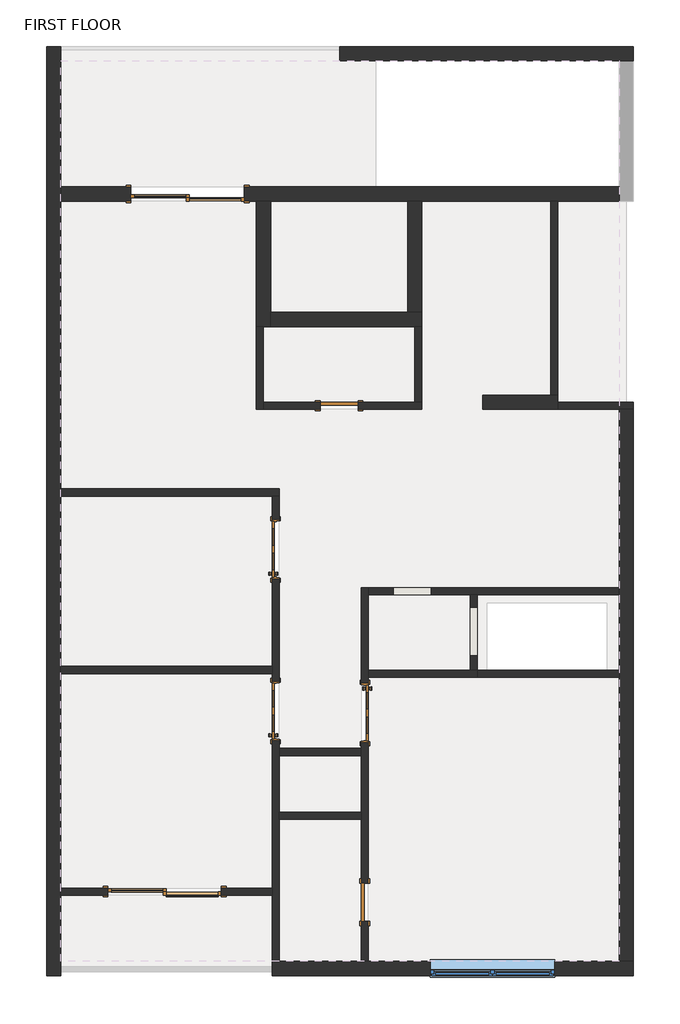
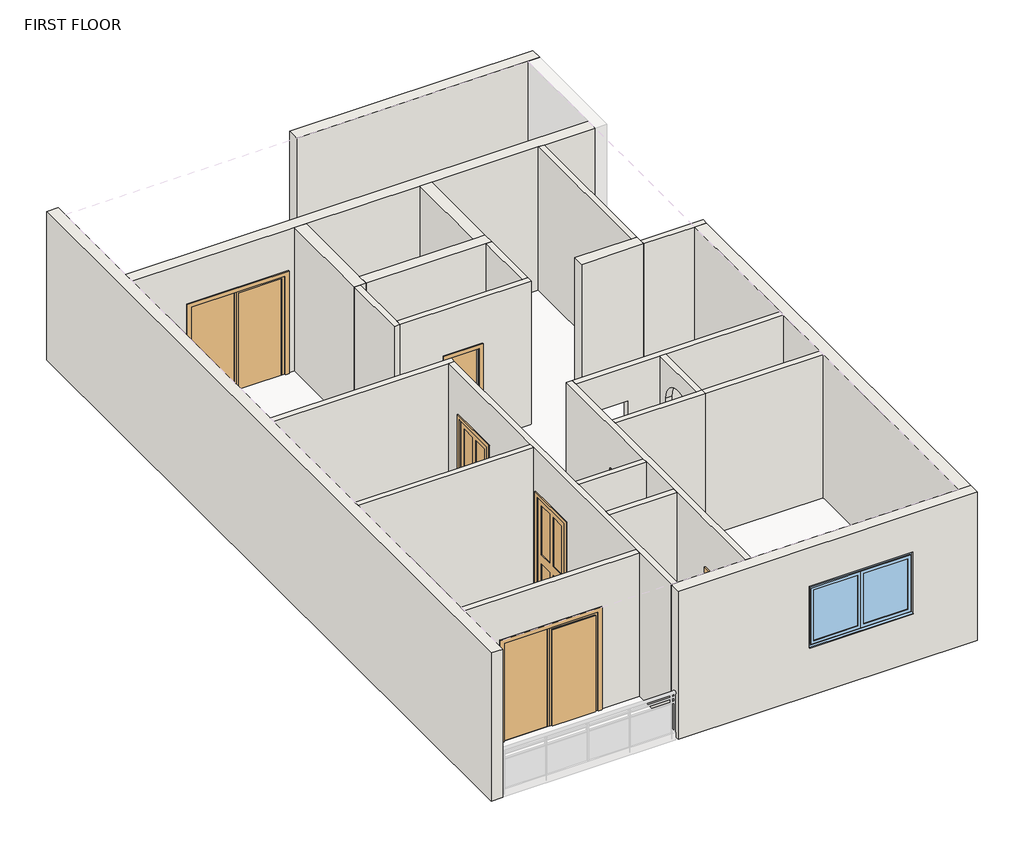
# One storey, part 1 of 2: 25 walls, 7 doors, 1 window.
"""IFC4 building model written with IfcOpenShell, lengths in millimetres."""

from ifc_helpers import new_model, si_unit, point, frame, frame_2d, origin, place, context, project, spatial, polyline, circle_curve, trimmed, segment, composite_curve, outline, extrude, faceted_brep, transform, mapped, element, save
from components import door_d4d75d1e, door_166d4031, door_c2926031, single_flush_bathroom_door_2_x_7_d2bb450e, w2_w2_7b90d420

model = new_model("IFC4")

# Units and contexts
model_context = context("Model", 3, world=origin())
ifc_project = project(units=[si_unit("LENGTHUNIT", "METRE", prefix="MILLI")], contexts=[model_context])

# Site, building, storey
site = spatial("IfcSite", under=ifc_project)
building = spatial("IfcBuilding", under=site)
storey = spatial("IfcBuildingStorey", under=building, Name="FIRST FLOOR", Elevation=3352.8)

# Doors
placement = place(None, origin())
door_shape = door_d4d75d1e(model_context)
element("IfcDoor", 1, ObjectType="Door-Double-Sliding : 72\" x 84\"", at=placement, inside=storey, context=model_context, shape_type="MappedRepresentation", body=[
    mapped(door_shape, transform((-16100.4229553, 5649.1964313, 3352.8), x_axis=(-1.0, 0.0, 0.0), y_axis=(0.0, -1.0, 0.0), z_axis=(0.0, 0.0, 1.0))),
])
door_2_shape = door_166d4031(model_context)
element("IfcDoor", 2, ObjectType="Door-Double-Sliding : 72\" x 84\"", at=placement, inside=storey, context=model_context, shape_type="MappedRepresentation", body=[
    mapped(door_2_shape, transform((-16471.8979553, -5583.9535687, 3352.8), x_axis=(-1.0, 0.0, 0.0), y_axis=(0.0, -1.0, 0.0), z_axis=(0.0, 0.0, 1.0))),
])
door_3_shape = door_c2926031(model_context)
element("IfcDoor", 3, ObjectType="Door-Interior-Single-4_Panel-Wood : 36\" x 84\"", at=placement, inside=storey, context=model_context, shape_type="MappedRepresentation", body=[
    mapped(door_3_shape, transform((-13246.0979553, -2834.4035687, 3352.8), x_axis=(0.0, -1.0, 0.0), y_axis=(1.0, 0.0, 0.0), z_axis=(0.0, 0.0, 1.0))),
])
element("IfcDoor", 4, ObjectType="Door-Interior-Single-4_Panel-Wood : 36\" x 84\"", at=placement, inside=storey, context=model_context, shape_type="MappedRepresentation", body=[
    mapped(door_3_shape, transform((-14687.5479553, -199.1535687, 3352.8), x_axis=(0.0, 1.0, 0.0), y_axis=(-1.0, 0.0, 0.0), z_axis=(0.0, 0.0, 1.0))),
])
element("IfcDoor", 5, ObjectType="Door-Interior-Single-4_Panel-Wood : 36\" x 84\"", at=placement, inside=storey, context=model_context, shape_type="MappedRepresentation", body=[
    mapped(door_3_shape, transform((-14687.5479553, -2802.6535687, 3352.8), x_axis=(0.0, 1.0, 0.0), y_axis=(-1.0, 0.0, 0.0), z_axis=(0.0, 0.0, 1.0))),
])
single_flush_bathroom_door_2_x_7_shape = single_flush_bathroom_door_2_x_7_d2bb450e(model_context)
element("IfcDoor", 6, ObjectType="Single-Flush : BATHROOM DOOR 2' X 7'", at=placement, inside=storey, context=model_context, shape_type="MappedRepresentation", body=[
    mapped(single_flush_bathroom_door_2_x_7_shape, transform((-13249.2729553, -5882.4035687, 3352.8), x_axis=(0.0, 1.0, 0.0), y_axis=(-1.0, 0.0, 0.0), z_axis=(0.0, 0.0, 1.0))),
])
element("IfcDoor", 7, ObjectType="Single-Flush : BATHROOM DOOR 2' X 7'", at=placement, inside=storey, context=model_context, shape_type="MappedRepresentation", body=[
    mapped(single_flush_bathroom_door_2_x_7_shape, transform((-13662.0229553, 2112.2464313, 3352.8), x_axis=(1.0, 0.0, 0.0), y_axis=(0.0, 1.0, 0.0), z_axis=(0.0, 0.0, 1.0))),
])

# Walls
element("IfcWall", 8, ObjectType="EXTERIOR WALL 9\"", at=placement, inside=storey, context=model_context, shape_type="Brep", body=[
    faceted_brep([(-13649.3229553, 7668.4964313, 3352.8), (-9153.5229553, 7668.4964313, 3352.8), (-8924.9229553, 7668.4964313, 3352.8), (-8924.9229553, 7668.4964313, 6400.8), (-9153.5229553, 7668.4964313, 6400.8), (-13649.3229553, 7668.4964313, 6400.8), (-13649.3229553, 7897.0964313, 3352.8), (-13649.3229553, 7897.0964313, 6400.8), (-8924.9229553, 7897.0964313, 6400.8), (-8924.9229553, 7897.0964313, 3352.8)], [[[0, 1, 2, 3, 4, 5]], [[6, 7, 8, 9]], [[2, 1, 0, 6, 9]], [[5, 4, 3, 8, 7]], [[0, 5, 7, 6]], [[3, 2, 9, 8]]]),
])
element("IfcWall", 9, ObjectType="EXTERIOR WALL 9\"", at=placement, inside=storey, context=model_context, shape_type="Brep", body=[
    faceted_brep([(-18373.7229553, 7897.0964313, 3352.8), (-18373.7229553, -7063.5035687, 3352.8), (-18373.7229553, -7063.5035687, 6400.8), (-18373.7229553, 7897.0964313, 6400.8), (-18145.1229553, 7897.0964313, 3352.8), (-18145.1229553, 7897.0964313, 6400.8), (-18145.1229553, 5636.4964313, 6400.8), (-18145.1229553, 5407.8964313, 6400.8), (-18145.1229553, 772.3964313, 6400.8), (-18145.1229553, 658.0964313, 6400.8), (-18145.1229553, -2085.1035687, 6400.8), (-18145.1229553, -2199.4035687, 6400.8), (-18145.1229553, -5653.8035687, 6400.8), (-18145.1229553, -5768.1035687, 6400.8), (-18145.1229553, -7063.5035687, 6400.8), (-18145.1229553, -7063.5035687, 3352.8), (-18145.1229553, -5768.1035687, 3352.8), (-18145.1229553, -5653.8035687, 3352.8), (-18145.1229553, -2199.4035687, 3352.8), (-18145.1229553, -2085.1035687, 3352.8), (-18145.1229553, 658.0964313, 3352.8), (-18145.1229553, 772.3964313, 3352.8), (-18145.1229553, 5407.8964313, 3352.8), (-18145.1229553, 5636.4964313, 3352.8)], [[[0, 1, 2, 3]], [[4, 5, 6, 7, 8, 9, 10, 11, 12, 13, 14, 15, 16, 17, 18, 19, 20, 21, 22, 23]], [[1, 0, 4, 23, 22, 21, 20, 19, 18, 17, 16, 15]], [[2, 1, 15, 14]], [[3, 2, 14, 13, 12, 11, 10, 9, 8, 7, 6, 5]], [[0, 3, 5, 4]]]),
])
element("IfcWall", 10, ObjectType="EXTERIOR WALL 9\"", at=placement, inside=storey, context=model_context, shape_type="Brep", body=[
    faceted_brep([(-18145.1229553, 5407.8964313, 3352.8), (-17014.8229553, 5407.8964313, 3352.8), (-17014.8229553, 5407.8964313, 5486.4), (-15186.0229553, 5407.8964313, 5486.4), (-15186.0229553, 5407.8964313, 3352.8), (-14995.5229553, 5407.8964313, 3352.8), (-14766.9229553, 5407.8964313, 3352.8), (-12557.1229553, 5407.8964313, 3352.8), (-12328.5229553, 5407.8964313, 3352.8), (-10258.4229553, 5407.8964313, 3352.8), (-10144.1229553, 5407.8964313, 3352.8), (-9153.5229553, 5407.8964313, 3352.8), (-9153.5229553, 5407.8964313, 6400.8), (-10144.1229553, 5407.8964313, 6400.8), (-10258.4229553, 5407.8964313, 6400.8), (-12328.5229553, 5407.8964313, 6400.8), (-12557.1229553, 5407.8964313, 6400.8), (-14766.9229553, 5407.8964313, 6400.8), (-14995.5229553, 5407.8964313, 6400.8), (-18145.1229553, 5407.8964313, 6400.8), (-17014.8229553, 5636.4964313, 5486.4), (-17014.8229553, 5636.4964313, 3352.8), (-18145.1229553, 5636.4964313, 3352.8), (-18145.1229553, 5636.4964313, 6400.8), (-9153.5229553, 5636.4964313, 6400.8), (-9153.5229553, 5636.4964313, 3352.8), (-15186.0229553, 5636.4964313, 3352.8), (-15186.0229553, 5636.4964313, 5486.4)], [[[0, 1, 2, 3, 4, 5, 6, 7, 8, 9, 10, 11, 12, 13, 14, 15, 16, 17, 18, 19]], [[20, 21, 22, 23, 24, 25, 26, 27]], [[26, 25, 11, 10, 9, 8, 7, 6, 5, 4]], [[22, 21, 1, 0]], [[19, 18, 17, 16, 15, 14, 13, 12, 24, 23]], [[12, 11, 25, 24]], [[0, 19, 23, 22]], [[4, 3, 27, 26]], [[2, 1, 21, 20]], [[3, 2, 20, 27]]]),
])
element("IfcWall", 11, ObjectType="EXTERIOR WALL 9\"", at=placement, inside=storey, context=model_context, shape_type="Brep", body=[
    faceted_brep([(-14995.5229553, 5407.8964313, 3352.8), (-14995.5229553, 3388.5964313, 3352.8), (-14995.5229553, 3388.5964313, 6400.8), (-14995.5229553, 5407.8964313, 6400.8), (-14766.9229553, 5407.8964313, 3352.8), (-14766.9229553, 5407.8964313, 6400.8), (-14766.9229553, 3617.1964313, 6400.8), (-14766.9229553, 3388.5964313, 6400.8), (-14766.9229553, 3388.5964313, 3352.8), (-14766.9229553, 3617.1964313, 3352.8), (-14881.2229553, 3388.5964313, 3352.8), (-14881.2229553, 3388.5964313, 6400.8)], [[[0, 1, 2, 3]], [[4, 5, 6, 7, 8, 9]], [[1, 0, 4, 9, 8, 10]], [[3, 2, 11, 7, 6, 5]], [[0, 3, 5, 4]], [[2, 1, 10, 8, 7, 11]]]),
])
element("IfcWall", 12, ObjectType="EXTERIOR WALL 9\"", at=placement, inside=storey, context=model_context, shape_type="Brep", body=[
    faceted_brep([(-14766.9229553, 3388.5964313, 3352.8), (-12442.8229553, 3388.5964313, 3352.8), (-12328.5229553, 3388.5964313, 3352.8), (-12328.5229553, 3388.5964313, 6400.8), (-12442.8229553, 3388.5964313, 6400.8), (-14766.9229553, 3388.5964313, 6400.8), (-14766.9229553, 3617.1964313, 3352.8), (-14766.9229553, 3617.1964313, 6400.8), (-12557.1229553, 3617.1964313, 6400.8), (-12328.5229553, 3617.1964313, 6400.8), (-12328.5229553, 3617.1964313, 3352.8), (-12557.1229553, 3617.1964313, 3352.8)], [[[0, 1, 2, 3, 4, 5]], [[6, 7, 8, 9, 10, 11]], [[2, 1, 0, 6, 11, 10]], [[5, 4, 3, 9, 8, 7]], [[0, 5, 7, 6]], [[3, 2, 10, 9]]]),
])
element("IfcWall", 13, ObjectType="EXTERIOR WALL 9\"", at=placement, inside=storey, context=model_context, shape_type="SweptSolid", body=[
    extrude(outline(polyline([(-12328.5229553, 5407.8964313), (-12328.5229553, 3617.1964313), (-12557.1229553, 3617.1964313), (-12557.1229553, 5407.8964313), (-12328.5229553, 5407.8964313)])), frame((0.0, 0.0, 3352.8), z_axis=(0.0, 0.0, 1.0), x_axis=(1.0, 0.0, 0.0)), (0.0, 0.0, 1.0), 3048.0),
])
element("IfcWall", 14, ObjectType="EXTERIOR WALL 9\"", at=placement, inside=storey, context=model_context, shape_type="Brep", body=[
    faceted_brep([(-14741.5229553, -7063.5035687, 3352.8), (-8924.9229553, -7063.5035687, 3352.8), (-8924.9229553, -7063.5035687, 6400.8), (-14741.5229553, -7063.5035687, 6400.8), (-12196.8729553, -7063.5035687, 4352.8), (-12196.8729553, -7063.5035687, 5612.8), (-10186.8729553, -7063.5035687, 5612.8), (-10186.8729553, -7063.5035687, 4352.8), (-14741.5229553, -6834.9035687, 3352.8), (-14741.5229553, -6834.9035687, 6400.8), (-14627.2229553, -6834.9035687, 6400.8), (-13306.4229553, -6834.9035687, 6400.8), (-13192.1229553, -6834.9035687, 6400.8), (-9153.5229553, -6834.9035687, 6400.8), (-8924.9229553, -6834.9035687, 6400.8), (-8924.9229553, -6834.9035687, 3352.8), (-9153.5229553, -6834.9035687, 3352.8), (-13192.1229553, -6834.9035687, 3352.8), (-13306.4229553, -6834.9035687, 3352.8), (-14627.2229553, -6834.9035687, 3352.8), (-12196.8729553, -6834.9035687, 4352.8), (-10186.8729553, -6834.9035687, 4352.8), (-10186.8729553, -6834.9035687, 5612.8), (-12196.8729553, -6834.9035687, 5612.8)], [[[0, 1, 2, 3], [4, 5, 6, 7]], [[8, 9, 10, 11, 12, 13, 14, 15, 16, 17, 18, 19], [20, 21, 22, 23]], [[1, 0, 8, 19, 18, 17, 16, 15]], [[3, 2, 14, 13, 12, 11, 10, 9]], [[2, 1, 15, 14]], [[0, 3, 9, 8]], [[5, 4, 20, 23]], [[6, 5, 23, 22]], [[7, 6, 22, 21]], [[4, 7, 21, 20]]]),
])
element("IfcWall", 15, ObjectType="EXTERIOR WALL 9\"", at=placement, inside=storey, context=model_context, shape_type="Brep", body=[
    faceted_brep([(-8924.9229553, -6834.9035687, 3352.8), (-8924.9229553, 2055.0964313, 3352.8), (-8924.9229553, 2055.0964313, 6400.8), (-8924.9229553, -6834.9035687, 6400.8), (-9153.5229553, -6834.9035687, 3352.8), (-9153.5229553, -6834.9035687, 6400.8), (-9153.5229553, -2262.9035687, 6400.8), (-9153.5229553, -2148.6035687, 6400.8), (-9153.5229553, -929.4035687, 6400.8), (-9153.5229553, -815.1035687, 6400.8), (-9153.5229553, 2055.0964313, 6400.8), (-9153.5229553, 2055.0964313, 3352.8), (-9153.5229553, -815.1035687, 3352.8), (-9153.5229553, -929.4035687, 3352.8), (-9153.5229553, -2148.6035687, 3352.8), (-9153.5229553, -2262.9035687, 3352.8)], [[[0, 1, 2, 3]], [[4, 5, 6, 7, 8, 9, 10, 11, 12, 13, 14, 15]], [[1, 0, 4, 15, 14, 13, 12, 11]], [[3, 2, 10, 9, 8, 7, 6, 5]], [[0, 3, 5, 4]], [[2, 1, 11, 10]]]),
])
element("IfcWall", 16, ObjectType="EXTERIOR WALL 9\"", at=placement, inside=storey, context=model_context, shape_type="Brep", body=[
    faceted_brep([(-11350.6229553, 2055.0964313, 3352.8), (-10144.1229553, 2055.0964313, 3352.8), (-10144.1229553, 2055.0964313, 6400.8), (-11350.6229553, 2055.0964313, 6400.8), (-11350.6229553, 2283.6964313, 3352.8), (-11350.6229553, 2283.6964313, 6400.8), (-10258.4229553, 2283.6964313, 6400.8), (-10144.1229553, 2283.6964313, 6400.8), (-10144.1229553, 2283.6964313, 3352.8), (-10258.4229553, 2283.6964313, 3352.8), (-10144.1229553, 2169.3964313, 3352.8), (-10144.1229553, 2169.3964313, 6400.8)], [[[0, 1, 2, 3]], [[4, 5, 6, 7, 8, 9]], [[1, 0, 4, 9, 8, 10]], [[3, 2, 11, 7, 6, 5]], [[0, 3, 5, 4]], [[2, 1, 10, 8, 7, 11]]]),
])
element("IfcWall", 17, ObjectType="INTERIOR WALL 4.5\"", at=placement, inside=storey, context=model_context, shape_type="Brep", body=[
    faceted_brep([(-18145.1229553, 658.0964313, 3352.8), (-14741.5229553, 658.0964313, 3352.8), (-14627.2229553, 658.0964313, 3352.8), (-14627.2229553, 658.0964313, 6400.8), (-14741.5229553, 658.0964313, 6400.8), (-18145.1229553, 658.0964313, 6400.8), (-18145.1229553, 772.3964313, 3352.8), (-18145.1229553, 772.3964313, 6400.8), (-14627.2229553, 772.3964313, 6400.8), (-14627.2229553, 772.3964313, 3352.8)], [[[0, 1, 2, 3, 4, 5]], [[6, 7, 8, 9]], [[2, 1, 0, 6, 9]], [[5, 4, 3, 8, 7]], [[0, 5, 7, 6]], [[3, 2, 9, 8]]]),
])
element("IfcWall", 18, ObjectType="INTERIOR WALL 4.5\"", at=placement, inside=storey, context=model_context, shape_type="Brep", body=[
    faceted_brep([(-14741.5229553, -6834.9035687, 6400.8), (-14741.5229553, -5768.1035687, 6400.8), (-14741.5229553, -5653.8035687, 6400.8), (-14741.5229553, -2199.4035687, 6400.8), (-14741.5229553, -2085.1035687, 6400.8), (-14741.5229553, 658.0964313, 6400.8), (-14741.5229553, 658.0964313, 3352.8), (-14741.5229553, 283.4464313, 3352.8), (-14741.5229553, 283.4464313, 5511.8), (-14741.5229553, -681.7535687, 5511.8), (-14741.5229553, -681.7535687, 3352.8), (-14741.5229553, -2085.1035687, 3352.8), (-14741.5229553, -2199.4035687, 3352.8), (-14741.5229553, -2320.0535687, 3352.8), (-14741.5229553, -2320.0535687, 5511.8), (-14741.5229553, -3285.2535687, 5511.8), (-14741.5229553, -3285.2535687, 3352.8), (-14741.5229553, -5653.8035687, 3352.8), (-14741.5229553, -5768.1035687, 3352.8), (-14741.5229553, -6834.9035687, 3352.8), (-14627.2229553, 658.0964313, 6400.8), (-14627.2229553, -3405.9035687, 6400.8), (-14627.2229553, -3520.2035687, 6400.8), (-14627.2229553, -4434.6035687, 6400.8), (-14627.2229553, -4548.9035687, 6400.8), (-14627.2229553, -6834.9035687, 6400.8), (-14627.2229553, -6834.9035687, 3352.8), (-14627.2229553, -4548.9035687, 3352.8), (-14627.2229553, -4434.6035687, 3352.8), (-14627.2229553, -3520.2035687, 3352.8), (-14627.2229553, -3405.9035687, 3352.8), (-14627.2229553, -3285.2535687, 3352.8), (-14627.2229553, -3285.2535687, 5511.8), (-14627.2229553, -2320.0535687, 5511.8), (-14627.2229553, -2320.0535687, 3352.8), (-14627.2229553, -681.7535687, 3352.8), (-14627.2229553, -681.7535687, 5511.8), (-14627.2229553, 283.4464313, 5511.8), (-14627.2229553, 283.4464313, 3352.8), (-14627.2229553, 658.0964313, 3352.8)], [[[0, 1, 2, 3, 4, 5, 6, 7, 8, 9, 10, 11, 12, 13, 14, 15, 16, 17, 18, 19]], [[20, 21, 22, 23, 24, 25, 26, 27, 28, 29, 30, 31, 32, 33, 34, 35, 36, 37, 38, 39]], [[6, 39, 38, 7]], [[26, 19, 18, 17, 16, 31, 30, 29, 28, 27]], [[10, 35, 34, 13, 12, 11]], [[5, 4, 3, 2, 1, 0, 25, 24, 23, 22, 21, 20]], [[6, 5, 20, 39]], [[0, 19, 26, 25]], [[37, 8, 7, 38]], [[8, 37, 36, 9]], [[9, 36, 35, 10]], [[33, 14, 13, 34]], [[14, 33, 32, 15]], [[15, 32, 31, 16]]]),
])
element("IfcWall", 19, ObjectType="INTERIOR WALL 4.5\"", at=placement, inside=storey, context=model_context, shape_type="SweptSolid", body=[
    extrude(outline(polyline([(-14741.5229553, -2199.4035687), (-18145.1229553, -2199.4035687), (-18145.1229553, -2085.1035687), (-14741.5229553, -2085.1035687), (-14741.5229553, -2199.4035687)])), frame((0.0, 0.0, 3352.8), z_axis=(0.0, 0.0, 1.0), x_axis=(1.0, 0.0, 0.0)), (0.0, 0.0, 1.0), 3048.0),
])
element("IfcWall", 20, ObjectType="INTERIOR WALL 4.5\"", at=placement, inside=storey, context=model_context, shape_type="SweptSolid", body=[
    extrude(outline(polyline([(3352.8, -18145.1229553), (3352.8, -17386.2979553), (5486.4, -17386.2979553), (5486.4, -15557.4979553), (3352.8, -15557.4979553), (3352.8, -14741.5229553), (6400.8, -14741.5229553), (6400.8, -18145.1229553), (3352.8, -18145.1229553)])), frame((0.0, -5768.1035687, 0.0), z_axis=(0.0, 1.0, 0.0), x_axis=(0.0, 0.0, 1.0)), (0.0, 0.0, 1.0), 114.3),
])
element("IfcWall", 21, ObjectType="INTERIOR WALL 4.5\"", at=placement, inside=storey, context=model_context, shape_type="Brep", body=[
    faceted_brep([(-13192.1229553, -5577.6035687, 5384.8), (-13192.1229553, -5577.6035687, 3352.8), (-13192.1229553, -3317.0035687, 3352.8), (-13192.1229553, -3317.0035687, 5511.8), (-13192.1229553, -2351.8035687, 5511.8), (-13192.1229553, -2351.8035687, 3352.8), (-13192.1229553, -2262.9035687, 3352.8), (-13192.1229553, -2148.6035687, 3352.8), (-13192.1229553, -929.4035687, 3352.8), (-13192.1229553, -815.1035687, 3352.8), (-13192.1229553, -815.1035687, 6400.8), (-13192.1229553, -929.4035687, 6400.8), (-13192.1229553, -2148.6035687, 6400.8), (-13192.1229553, -2262.9035687, 6400.8), (-13192.1229553, -6834.9035687, 6400.8), (-13192.1229553, -6834.9035687, 3352.8), (-13192.1229553, -6187.2035687, 3352.8), (-13192.1229553, -6187.2035687, 5384.8), (-13306.4229553, -3317.0035687, 3352.8), (-13306.4229553, -3405.9035687, 3352.8), (-13306.4229553, -3520.2035687, 3352.8), (-13306.4229553, -4434.6035687, 3352.8), (-13306.4229553, -4548.9035687, 3352.8), (-13306.4229553, -5577.6035687, 3352.8), (-13306.4229553, -5577.6035687, 5384.8), (-13306.4229553, -6187.2035687, 5384.8), (-13306.4229553, -6187.2035687, 3352.8), (-13306.4229553, -6834.9035687, 3352.8), (-13306.4229553, -6834.9035687, 6400.8), (-13306.4229553, -4548.9035687, 6400.8), (-13306.4229553, -4434.6035687, 6400.8), (-13306.4229553, -3520.2035687, 6400.8), (-13306.4229553, -3405.9035687, 6400.8), (-13306.4229553, -815.1035687, 6400.8), (-13306.4229553, -815.1035687, 3352.8), (-13306.4229553, -2351.8035687, 3352.8), (-13306.4229553, -2351.8035687, 5511.8), (-13306.4229553, -3317.0035687, 5511.8)], [[[0, 1, 2, 3, 4, 5, 6, 7, 8, 9, 10, 11, 12, 13, 14, 15, 16, 17]], [[18, 19, 20, 21, 22, 23, 24, 25, 26, 27, 28, 29, 30, 31, 32, 33, 34, 35, 36, 37]], [[34, 9, 8, 7, 6, 5, 35]], [[16, 15, 27, 26]], [[2, 1, 23, 22, 21, 20, 19, 18]], [[14, 13, 12, 11, 10, 33, 32, 31, 30, 29, 28]], [[15, 14, 28, 27]], [[10, 9, 34, 33]], [[37, 3, 2, 18]], [[3, 37, 36, 4]], [[4, 36, 35, 5]], [[24, 23, 1, 0]], [[25, 24, 0, 17]], [[26, 25, 17, 16]]]),
])
element("IfcWall", 22, ObjectType="INTERIOR WALL 4.5\"", at=placement, inside=storey, context=model_context, shape_type="SweptSolid", body=[
    extrude(outline(polyline([(-14627.2229553, -3405.9035687), (-13306.4229553, -3405.9035687), (-13306.4229553, -3520.2035687), (-14627.2229553, -3520.2035687), (-14627.2229553, -3405.9035687)])), frame((0.0, 0.0, 3352.8), z_axis=(0.0, 0.0, 1.0), x_axis=(1.0, 0.0, 0.0)), (0.0, 0.0, 1.0), 3048.0),
])
element("IfcWall", 23, ObjectType="INTERIOR WALL 4.5\"", at=placement, inside=storey, context=model_context, shape_type="SweptSolid", body=[
    extrude(outline(polyline([(-13306.4229553, -4548.9035687), (-14627.2229553, -4548.9035687), (-14627.2229553, -4434.6035687), (-13306.4229553, -4434.6035687), (-13306.4229553, -4548.9035687)])), frame((0.0, 0.0, 3352.8), z_axis=(0.0, 0.0, 1.0), x_axis=(1.0, 0.0, 0.0)), (0.0, 0.0, 1.0), 3048.0),
])
element("IfcWall", 24, ObjectType="INTERIOR WALL 4.5\"", at=placement, inside=storey, context=model_context, shape_type="Brep", body=[
    faceted_brep([(-13192.1229553, -929.4035687, 3352.8), (-11553.8229553, -929.4035687, 3352.8), (-11439.5229553, -929.4035687, 3352.8), (-9153.5229553, -929.4035687, 3352.8), (-9153.5229553, -929.4035687, 6400.8), (-11439.5229553, -929.4035687, 6400.8), (-11553.8229553, -929.4035687, 6400.8), (-13192.1229553, -929.4035687, 6400.8), (-12792.0729553, -929.4035687, 3657.6), (-12792.0729553, -929.4035687, 5689.6), (-12182.4729553, -929.4035687, 5689.6), (-12182.4729553, -929.4035687, 3657.6), (-13192.1229553, -815.1035687, 3352.8), (-13192.1229553, -815.1035687, 6400.8), (-9153.5229553, -815.1035687, 6400.8), (-9153.5229553, -815.1035687, 3352.8), (-12792.0729553, -815.1035687, 3657.6), (-12182.4729553, -815.1035687, 3657.6), (-12182.4729553, -815.1035687, 5689.6), (-12792.0729553, -815.1035687, 5689.6)], [[[0, 1, 2, 3, 4, 5, 6, 7], [8, 9, 10, 11]], [[12, 13, 14, 15], [16, 17, 18, 19]], [[3, 2, 1, 0, 12, 15]], [[7, 6, 5, 4, 14, 13]], [[0, 7, 13, 12]], [[4, 3, 15, 14]], [[17, 16, 8, 11]], [[18, 17, 11, 10]], [[19, 18, 10, 9]], [[16, 19, 9, 8]]]),
])
element("IfcWall", 25, ObjectType="INTERIOR WALL 4.5\"", at=placement, inside=storey, context=model_context, shape_type="Brep", body=[
    faceted_brep([(-13192.1229553, -2262.9035687, 3352.8), (-11439.5229553, -2262.9035687, 3352.8), (-11439.5229553, -2262.9035687, 6400.8), (-13192.1229553, -2262.9035687, 6400.8), (-13192.1229553, -2148.6035687, 3352.8), (-13192.1229553, -2148.6035687, 6400.8), (-11553.8229553, -2148.6035687, 6400.8), (-11439.5229553, -2148.6035687, 6400.8), (-11439.5229553, -2148.6035687, 3352.8), (-11553.8229553, -2148.6035687, 3352.8)], [[[0, 1, 2, 3]], [[4, 5, 6, 7, 8, 9]], [[1, 0, 4, 9, 8]], [[3, 2, 7, 6, 5]], [[0, 3, 5, 4]], [[2, 1, 8, 7]]]),
])
element("IfcWall", 26, ObjectType="INTERIOR WALL 4.5\"", at=placement, inside=storey, context=model_context, shape_type="SweptSolid", body=[
    extrude(outline(polyline([(-2148.6035687, 3352.8), (-2148.6035687, 6400.8), (-929.4035687, 6400.8), (-929.4035687, 3352.8), (-2148.6035687, 3352.8)]), holes=[composite_curve([segment(polyline([(-1910.1162217, 3535.9698034), (-1135.4162217, 3535.9698034), (-1135.4162217, 5656.8698034)]), True, "CONTINUOUS"), segment(trimmed(circle_curve(frame_2d((-1522.7662217, 5656.8698034)), 387.35), [point((-1135.4162217, 5656.8698034))], [point((-1910.1162217, 5656.8698034))], True, "CARTESIAN"), True, "CONTINUOUS"), segment(polyline([(-1910.1162217, 5656.8698034), (-1910.1162217, 3535.9698034)]), True, "CONTINUOUS")], self_intersect=False)]), frame((-11553.8229553, 0.0, 0.0), z_axis=(1.0, 0.0, 0.0), x_axis=(0.0, 1.0, 0.0)), (0.0, 0.0, 1.0), 114.3),
])
element("IfcWall", 27, ObjectType="INTERIOR WALL 4.5\"", at=placement, inside=storey, context=model_context, shape_type="SweptSolid", body=[
    extrude(outline(polyline([(-11439.5229553, -2148.6035687), (-9153.5229553, -2148.6035687), (-9153.5229553, -2262.9035687), (-11439.5229553, -2262.9035687), (-11439.5229553, -2148.6035687)])), frame((0.0, 0.0, 3352.8), z_axis=(0.0, 0.0, 1.0), x_axis=(1.0, 0.0, 0.0)), (0.0, 0.0, 1.0), 3048.0),
])
element("IfcWall", 28, ObjectType="INTERIOR WALL 4.5\"", at=placement, inside=storey, context=model_context, shape_type="Brep", body=[
    faceted_brep([(-14995.5229553, 3388.5964313, 3352.8), (-14995.5229553, 2055.0964313, 3352.8), (-14995.5229553, 2055.0964313, 6400.8), (-14995.5229553, 3388.5964313, 6400.8), (-14881.2229553, 3388.5964313, 3352.8), (-14881.2229553, 3388.5964313, 6400.8), (-14881.2229553, 2169.3964313, 6400.8), (-14881.2229553, 2055.0964313, 6400.8), (-14881.2229553, 2055.0964313, 3352.8), (-14881.2229553, 2169.3964313, 3352.8)], [[[0, 1, 2, 3]], [[4, 5, 6, 7, 8, 9]], [[1, 0, 4, 9, 8]], [[3, 2, 7, 6, 5]], [[0, 3, 5, 4]], [[2, 1, 8, 7]]]),
])
element("IfcWall", 29, ObjectType="INTERIOR WALL 4.5\"", at=placement, inside=storey, context=model_context, shape_type="Brep", body=[
    faceted_brep([(-13357.2229553, 2055.0964313, 5384.8), (-13357.2229553, 2055.0964313, 3352.8), (-12328.5229553, 2055.0964313, 3352.8), (-12328.5229553, 2055.0964313, 6400.8), (-14881.2229553, 2055.0964313, 6400.8), (-14881.2229553, 2055.0964313, 3352.8), (-13966.8229553, 2055.0964313, 3352.8), (-13966.8229553, 2055.0964313, 5384.8), (-12328.5229553, 2169.3964313, 3352.8), (-12442.8229553, 2169.3964313, 3352.8), (-13357.2229553, 2169.3964313, 3352.8), (-13357.2229553, 2169.3964313, 5384.8), (-13966.8229553, 2169.3964313, 5384.8), (-13966.8229553, 2169.3964313, 3352.8), (-14881.2229553, 2169.3964313, 3352.8), (-14881.2229553, 2169.3964313, 6400.8), (-12442.8229553, 2169.3964313, 6400.8), (-12328.5229553, 2169.3964313, 6400.8)], [[[0, 1, 2, 3, 4, 5, 6, 7]], [[8, 9, 10, 11, 12, 13, 14, 15, 16, 17]], [[6, 5, 14, 13]], [[2, 1, 10, 9, 8]], [[4, 3, 17, 16, 15]], [[5, 4, 15, 14]], [[3, 2, 8, 17]], [[11, 10, 1, 0]], [[12, 11, 0, 7]], [[13, 12, 7, 6]]]),
])
element("IfcWall", 30, ObjectType="INTERIOR WALL 4.5\"", at=placement, inside=storey, context=model_context, shape_type="SweptSolid", body=[
    extrude(outline(polyline([(-12328.5229553, 3388.5964313), (-12328.5229553, 2169.3964313), (-12442.8229553, 2169.3964313), (-12442.8229553, 3388.5964313), (-12328.5229553, 3388.5964313)])), frame((0.0, 0.0, 3352.8), z_axis=(0.0, 0.0, 1.0), x_axis=(1.0, 0.0, 0.0)), (0.0, 0.0, 1.0), 3048.0),
])
element("IfcWall", 31, ObjectType="INTERIOR WALL 4.5\"", at=placement, inside=storey, context=model_context, shape_type="SweptSolid", body=[
    extrude(outline(polyline([(-10258.4229553, 2283.6964313), (-10258.4229553, 5407.8964313), (-10144.1229553, 5407.8964313), (-10144.1229553, 2283.6964313), (-10258.4229553, 2283.6964313)])), frame((0.0, 0.0, 3352.8), z_axis=(0.0, 0.0, 1.0), x_axis=(1.0, 0.0, 0.0)), (0.0, 0.0, 1.0), 3048.0),
])
element("IfcWall", 32, ObjectType="INTERIOR WALL 4.5\"", at=placement, inside=storey, context=model_context, shape_type="Brep", body=[
    faceted_brep([(-10144.1229553, 2055.0964313, 3352.8), (-9153.5229553, 2055.0964313, 3352.8), (-8924.9229553, 2055.0964313, 3352.8), (-8924.9229553, 2055.0964313, 6400.8), (-9153.5229553, 2055.0964313, 6400.8), (-10144.1229553, 2055.0964313, 6400.8), (-10144.1229553, 2169.3964313, 3352.8), (-10144.1229553, 2169.3964313, 6400.8), (-8924.9229553, 2169.3964313, 6400.8), (-8924.9229553, 2169.3964313, 3352.8)], [[[0, 1, 2, 3, 4, 5]], [[6, 7, 8, 9]], [[2, 1, 0, 6, 9]], [[5, 4, 3, 8, 7]], [[0, 5, 7, 6]], [[3, 2, 9, 8]]]),
])

# Window
w2_w2_shape = w2_w2_7b90d420(model_context)
element("IfcWindow", 33, ObjectType="w2 : w2", at=placement, inside=storey, context=model_context, shape_type="MappedRepresentation", body=[
    mapped(w2_w2_shape, transform((-11191.8729553, -6949.2035687, 3352.8), x_axis=(1.0, 0.0, 0.0), y_axis=(0.0, 1.0, 0.0), z_axis=(0.0, 0.0, 1.0))),
])

save(model, "model.ifc")

# Revit data of these elements
# Type "Door-Double-Sliding : 72\" x 84\""
#   Type Mark = "9"
#   Construction Type Id = "opn-d45"
#   Assembly Code = "C1020"
#   Analytic Construction = "Wood frame, double glass door "
#   Thickness = 0' - 2"
#   Thermal Resistance (R) = 1.8150 (h·ft²·°F)/BTU
#   Heat Transfer Coefficient (U) = 0.5510 BTU/(h·ft²·°F)
#   Height = 7' - 0"
#   Rail Width = 0' - 2"
#   Stiles = 0' - 2"
#   Trim Projection Ext = 0' - 1"
#   Trim Projection Int = 0' - 1"
#   Trim Width = 0' - 3"
#   Width = 6' - 0"
#   Define Thermal Properties by = 1
#   Glazing = Glass
#   Panel Material = Wood - Birch - Solid Stained Light Low Gloss
#   Trim Material = Paint - Sienna
#   Visual Light Transmittance = 0
#   Solar Heat Gain Coefficient = 0
#   Function = (empty or 0)
#   Wall Closure = (empty or 0)
# Type "Door-Interior-Single-4_Panel-Wood : 36\" x 84\""
#   Type Mark = "10"
#   Assembly Code = "C1020300"
#   Analytic Construction = "Wooden"
#   Top Rail = 0' - 4 11/16"
#   Thickness = 0' - 1 3/8"
#   Thermal Resistance (R) = 2.5876 (h·ft²·°F)/BTU
#   Swing Angle [instance default] = 90.00°
#   Stiles = 0' - 4 3/4"
#   Rough Width = 3' - 2"
#   Rough Height = 7' - 1"
#   Mullion = 0' - 4 1/2"
#   Lock Rail = 0' - 7 1/2"
#   Height = 7' - 0"
#   Width = 3' - 0"
#   Heat Transfer Coefficient (U) = 0.3865 BTU/(h·ft²·°F)
#   Bottom Rail = 0' - 9 1/8"
#   Trim Material = Cherry
#   Panel Material = Cherry
#   Frame Material = Cherry
#   Door Handle Material = Aluminum
#   Visual Light Transmittance = 0
#   Solar Heat Gain Coefficient = 0
#   Wall Closure = (empty or 0)
#   Function = (empty or 0)
# Type "Single-Flush : BATHROOM DOOR 2' X 7'"
#   Type Mark = "11"
#   Construction Type Id = "MDOOR"
#   Assembly Code = "C1020"
#   Analytic Construction = "Metal"
#   Thickness = 0' - 2"
#   Heat Transfer Coefficient (U) = 0.651978 BTU/(h·ft²·°F)
#   Height = 6' - 8"
#   Trim Projection Ext = 0' - 1"
#   Trim Projection Int = 0' - 1"
#   Trim Width = 0' - 3"
#   Width = 2' - 0"
#   Define Thermal Properties by = 1
#   Door Material = Door - Panel
#   Frame Material = Door - Frame
#   Visual Light Transmittance = 0
#   Solar Heat Gain Coefficient = 0
#   Function = (empty or 0)
#   Wall Closure = (empty or 0)
# Type "EXTERIOR WALL 9\""
#   Assembly Code = "B2010"
#   Layers, outside or top first: 0' - 9" "EXTERIOR WALL WHITE COLOUR" (function 1)
# Type "INTERIOR WALL 4.5\""
#   Assembly Code = "B2010"
#   Layers, outside or top first: 0' - 4 1/2" "EXTERIOR WALL WHITE COLOUR" (function 1)
# Type "w2 : w2"
#   Type Mark = "18"
#   Operation = "DoublePanelVertical"
#   Keynote = "16.05.01"
#   Analytic Construction = "<None>"
#   Rough Width = 6' - 7.13386"
#   Rough Height = 4' - 1.6063"
#   Rahmentiefe = 0' - 2.3622"
#   Rahmenhöhe unten = 0' - 3.14961"
#   Rahmehöhe oben = 0' - 3.14961"
#   Rahmenbreite = 0' - 2.3622"
#   Heat Transfer Coefficient (U) = 2.81836 BTU/(h·ft²·°F)
#   Height = 4' - 1.6063"
#   Flügeltiefe = 0' - 2.3622"
#   Flügelbreite = 0' - 2.3622"
#   Einbautiefe (von außen) [instance default] = 0' - 5.51181"
#   Width = 6' - 7.13386"
#   Kippflügel [instance default] = yes
#   Drehflügel im Grundriß darstellen [instance default] = no
#   Drehflügel [instance default] = yes
#   Define Thermal Properties by = 1
#   Rahmen [instance default] = none
#   Glas [instance default] = blue glass
#   Flügel [instance default] = WINDOW COLOUR WHITE
#   Fensterbank aussen [instance default] = WINDOW COLOUR WHITE
#   Fensterbank innen [instance default] = WINDOW COLOUR WHITE
#   Visual Light Transmittance = 0
#   Thermal Resistance (R) = 0
#   Solar Heat Gain Coefficient = 0
#   Wall Closure = (empty or 0)
# Elements 1, 2 (IfcDoor, "Door-Double-Sliding : 72\" x 84\"")
#   Phase Created = New Construction
#   Materials on its faces: "Paint - Sienna", "Wood - Birch - Solid Stained Light Low Gloss", "Glass"
# Elements 3, 4, 5 (IfcDoor, "Door-Interior-Single-4_Panel-Wood : 36\" x 84\"")
#   Swing Angle = 90.00°
#   Phase Created = New Construction
#   Materials on its faces: "Cherry", "Aluminum"
# Elements 6, 7 (IfcDoor, "Single-Flush : BATHROOM DOOR 2' X 7'")
#   Phase Created = New Construction
#   Materials on its faces: "Door - Frame", "Door - Panel"
# Elements 8, 9, 10, 11, 12, 13, 14, 15, 16 (IfcWall, "EXTERIOR WALL 9\"")
#   Top Offset = 0' - 0"
#   Base Offset = 0' - 0"
#   wall height = 10' - 0"
#   Phase Created = New Construction
#   Base Constraint = FIRST FLOOR
#   Top Constraint = SECOND FLR
#   Materials on its faces: "EXTERIOR WALL WHITE COLOUR"
# Elements 17, 18, 19, 20, 21, 22, 23, 24, 25, 26, 27, 28, 29, 30, 31, 32 (IfcWall, "INTERIOR WALL 4.5\"")
#   Top Offset = 0' - 0"
#   Base Offset = 0' - 0"
#   wall height = 10' - 0"
#   Phase Created = New Construction
#   Base Constraint = FIRST FLOOR
#   Top Constraint = SECOND FLR
#   Materials on its faces: "EXTERIOR WALL WHITE COLOUR"
# Element 33 (IfcWindow, "w2 : w2")
#   Mark = "2"
#   Einbautiefe (von außen) = 0' - 5.51181"
#   Kippflügel = yes
#   Drehflügel im Grundriß darstellen = no
#   Drehflügel = yes
#   Rahmen = none
#   Glas = blue glass
#   Flügel = WINDOW COLOUR WHITE
#   Fensterbank innen = WINDOW COLOUR WHITE
#   Fensterbank aussen = WINDOW COLOUR WHITE
#   Phase Created = New Construction
#   Materials on its faces: "WINDOW COLOUR WHITE", "blue glass"
# Materials
#   "Glass": class "Glass", colour RGB 0 128 192, transparency 0.75, Description = "Soda Lime Glass", Cost = 0
#   "Wood - Birch - Solid Stained Light Low Gloss": class "Wood", colour RGB 210 159 95, transparency 0, Cost = 0
#   "Paint - Sienna": colour RGB 118 70 51, transparency 0, Cost = 0
#   "Cherry": class "Wood", colour RGB 226 177 128, transparency 0, Description = "Prunus Serotina", Cost = 0
#   "Aluminum": class "Metal", colour RGB 247 247 247, transparency 0, Description = "Aluminum 6061", Cost = 0
#   "Door - Panel": class "Wood", colour RGB 210 159 95, transparency 0, Cost = 0
#   "Door - Frame": colour RGB 118 70 51, transparency 0, Cost = 0
#   "EXTERIOR WALL WHITE COLOUR": class "Generic", colour RGB 120 120 120, transparency 0, Cost = 0
#   "blue glass": class "System", colour RGB 0 0 255, transparency 0.75, Cost = 0
#   "WINDOW COLOUR WHITE": class "Generic", colour RGB 120 120 120, transparency 0, Cost = 0
